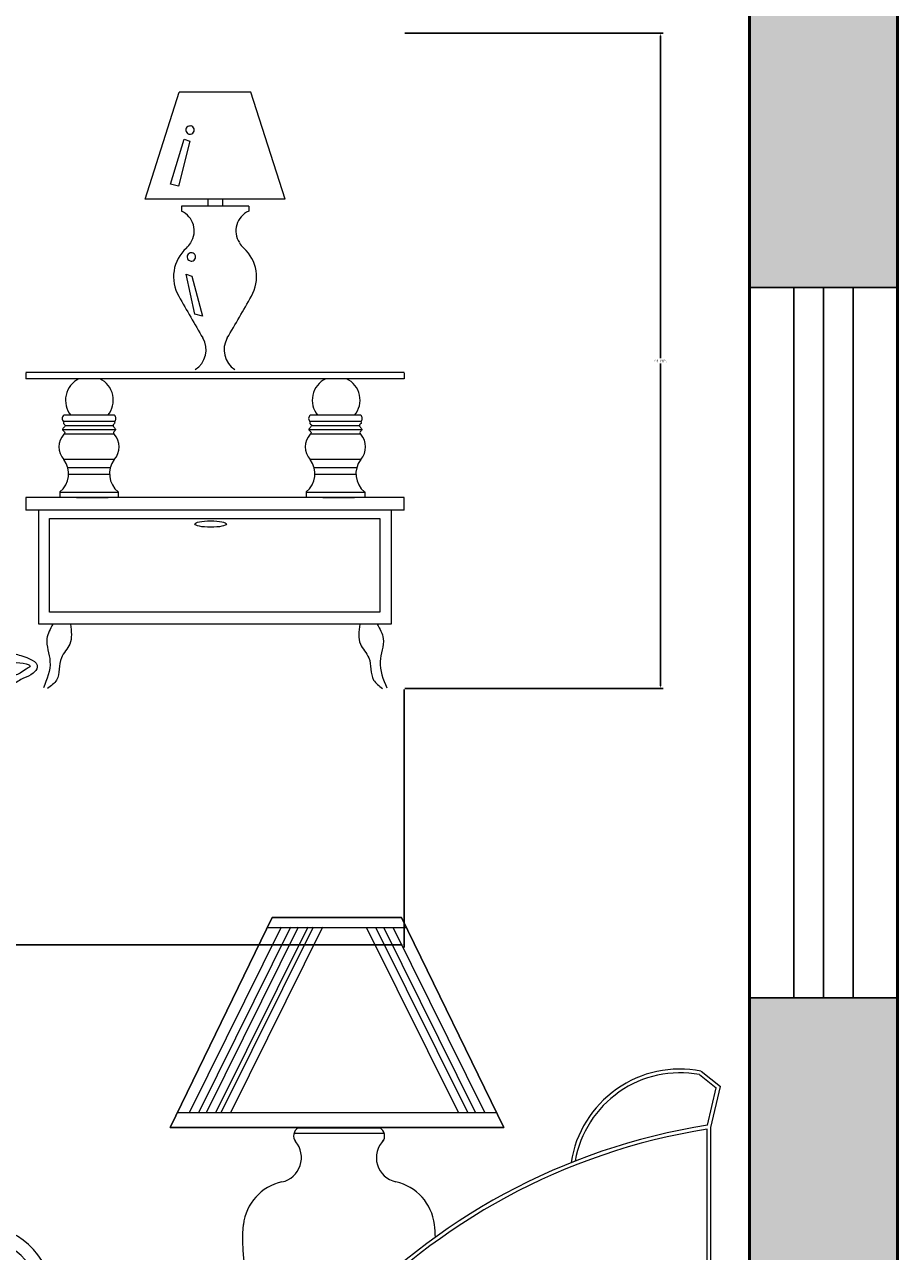
# Model space of a CAD drawing. Units: inches. Extents: x 1771 to 3025, y 319 to 889.
# Tile 23 of 35: x 2502 to 2561, y 703 to 786. Entities that reach past the tile are written whole.
import ezdxf

# ---------------------------------------------------------------- set-up
doc = ezdxf.new("R2010")
doc.units = ezdxf.units.IN
doc.header["$MEASUREMENT"] = 0
doc.set_wipeout_variables(frame=1)
for name, color, linetype, lineweight in [('A-ANNO-DIMS', 2, 'Continuous', 18), ('A-FURN', 8, 'Continuous', 18), ('A-GLAZ', 40, 'Continuous', 25), ('A-WALL', 7, 'Continuous', 50), ('A-WALL-PATT', 254, 'Continuous', 13)]:
    doc.layers.add(name, color=color, linetype=linetype, lineweight=lineweight)
doc.styles.get("Standard").update_dxf_attribs({"font": 'arial.ttf'})
doc.dimstyles.get("Standard").update_dxf_attribs({"dimtxt": 0.18, "dimasz": 0.18, "dimexe": 0.18, "dimexo": 0.0625, "dimgap": 0.09, "dimtad": 0, "dimtih": 1, "dimtoh": 1, "dimdec": 4, "dimzin": 0, "dimdsep": 46, "dimtxsty": 'Standard', "dimcen": 0.09, "dimadec": 0, "dimazin": 0, "dimtfac": 1, "dimtdec": 4, "dimtofl": 0, "dimtmove": 0, "dimatfit": 3, "dimfxl": 1, "dimtolj": 1, "dimtzin": 0, "dimarcsym": 0})

# ---------------------------------------------------------------- blocks, each defined once
blk = doc.blocks.new('A$C3F6F0378')
for p, q in [((2294.6, 774.2), (2348.7, 943.6)), ((2462.2, 943.6), (2348.7, 943.6)), ((2516.4, 774.2), (2462.2, 943.6)), ((2335.1, 797.8), (2356.3, 869.3)), ((2365.5, 866.2), (2347.3, 794.8)), ((2356.3, 869.3), (2365.5, 866.2)), ((2347.3, 794.8), (2335.1, 797.8)), ((2516.4, 774.2), (2294.6, 774.2)), ((2352.3, 763), (2352.3, 755.2)), ((2352.3, 763), (2352.3, 755.2)), ((2458.6, 763), (2352.3, 763)), ((2393.8, 774.2), (2393.8, 763)), ((2417.1, 763), (2393.8, 763)), ((2417.1, 774.2), (2417.1, 763)), ((2458.6, 763), (2458.6, 755.2)), ((2458.6, 763), (2458.6, 755.2)), ((2359.5, 655.6), (2368.6, 652.5)), ((2373.2, 592.3), (2359.5, 655.6)), ((2368.6, 652.5), (2385.4, 589.2)), ((2385.4, 589.2), (2373.2, 592.3)), ((2704.5, 500), (2106.1, 500)), ((2106.1, 499.7), (2106.1, 489.7)), ((2704.5, 490), (2106.1, 490)), ((2704.5, 499.7), (2704.5, 489.7)), ((2246.1, 432.2), (2166.1, 432.2)), ((2246.1, 432.2), (2166.1, 432.2)), ((2635.9, 432.2), (2555.9, 432.2)), ((2635.9, 432.2), (2555.9, 432.2)), ((2248, 409.3), (2164.1, 409.3)), ((2246.1, 422.2), (2166.1, 422.2)), ((2244.2, 415.4), (2167.9, 415.4)), ((2637.9, 409.3), (2554, 409.3)), ((2635.9, 422.2), (2555.9, 422.2)), ((2634.1, 415.4), (2557.7, 415.4)), ((2246.1, 402.2), (2166.1, 402.2)), ((2635.9, 402.2), (2555.9, 402.2)), ((2246.1, 362.2), (2166.1, 362.2)), ((2635.9, 362.2), (2555.9, 362.2)), ((2239.7, 349.2), (2172.4, 349.2)), ((2238.5, 338.7), (2173.6, 338.7)), ((2629.6, 349.2), (2562.2, 349.2)), ((2628.4, 338.7), (2563.5, 338.7)), ((2159.8, 311), (2159.8, 302.2)), ((2252.3, 311), (2252.3, 302.2)), ((2549.7, 311), (2549.7, 302.2)), ((2642.2, 311), (2642.2, 302.2)), ((2106.1, 302.2), (2106.1, 282.2)), ((2704.5, 302.2), (2106.1, 302.2)), ((2252.3, 310.3), (2159.8, 310.3)), ((2186.1, 302.2), (2226.1, 302.2)), ((2186.1, 302.2), (2236.1, 302.2)), ((2642.2, 310.3), (2549.7, 310.3)), ((2575.9, 302.2), (2615.9, 302.2)), ((2575.9, 302.2), (2625.9, 302.2)), ((2704.5, 282.2), (2704.5, 302.2)), ((2704.5, 282.2), (2106.1, 282.2)), ((2126.1, 282.2), (2126.1, 102.2)), ((2684.5, 102.2), (2684.5, 282.2)), ((2143.3, 268.9), (2666.3, 268.9)), ((2143.3, 120.8), (2143.3, 268.9)), ((2666.3, 268.9), (2666.3, 120.8)), ((2666.3, 120.8), (2143.3, 120.8)), ((2126.1, 102.2), (2684.5, 102.2))]:
    blk.add_line(p, q)
for centre, radius, start, end in [((2365.7, 883.6), 6.48, 168.6084, 233.2112), ((2365.7, 883.6), 6.49, 104.0344, 168.6084), ((2365.7, 883.5), 6.42, 233.2112, 255.9722), ((2366.1, 883.6), 6.51, 78.6968, 107.1924), ((2365.7, 883.8), 6.69, 255.9722, 278.2688), ((2365.7, 883.9), 6.81, 278.2688, 342.9026), ((2366.1, 883.7), 6.5, 50.1648, 78.6968), ((2366.2, 883.8), 6.35, 342.9026, 50.1648), ((2338.7, 724.1), 33.9, 326.6744, 66.3416), ((2472.2, 724.1), 33.9, 113.6584, 213.3256), ((2337, 722.3), 34.4, 312.0366, 330.6067), ((2473.8, 722.3), 34.4, 209.3933, 227.9634), ((2401.2, 651.2), 61.5, 132.0366, 209.8723), ((2367.7, 682.8), 6.48, 168.6084, 233.2112), ((2367.7, 682.8), 6.49, 104.0344, 168.6084), ((2368.1, 682.9), 6.51, 78.6968, 107.1924), ((2367.8, 683.1), 6.81, 278.2688, 342.9026), ((2368.1, 682.9), 6.5, 50.1648, 78.6968), ((2368.2, 683), 6.35, 342.9026, 50.1648), ((2409.6, 651.2), 61.5, 330.1277, 47.9634), ((2367.7, 682.8), 6.42, 233.2112, 255.9722), ((2367.8, 683), 6.69, 255.9722, 278.2688), ((11218.8, 5715.8), 10230.1, 209.87228, 210.29853), ((-6408, 5715.8), 10230.1, 329.70147, 330.12772), ((2353.9, 535.9), 37.3, 302.5427, 30.2985), ((2457, 535.9), 37.3, 149.7015, 237.4573), ((2206.6, 456.1), 37.8, 115.9414, 219.2084), ((2206.6, 456.1), 37.8, 320.7916, 64.0586), ((2597, 456.1), 37.8, 115.9414, 219.2084), ((2597, 456.1), 37.8, 320.7916, 64.0586), ((2169.8, 427.2), 6.24, 126.78, 233.22), ((2242.3, 427.2), 6.24, 306.78, 53.22), ((2559.7, 427.2), 6.24, 126.78, 233.22), ((2632.2, 427.2), 6.24, 306.78, 53.22), ((2188.1, 382.2), 29.7, 137.7452, 222.2548), ((2224, 382.2), 29.7, 317.7452, 42.2548), ((2577.9, 382.2), 29.7, 137.7452, 222.2548), ((2613.9, 382.2), 29.7, 317.7452, 42.2548), ((2136.7, 339.8), 37, 308.7547, 37.2668), ((2275.4, 339.8), 37, 142.7332, 231.2453), ((2526.5, 339.8), 37, 308.7547, 37.2668), ((2665.3, 339.8), 37, 142.7332, 231.2453)]:
    blk.add_arc(centre, radius, start, end)
blk.add_ellipse((2398.3, 260.1), major_axis=(25, 0), ratio=0.2)
for points, knots in [([(2166.1, 422.2), (2165.6, 421), (2164.6, 418.8), (2169.4, 417.1), (2166.2, 412.9), (2162.3, 408.7), (2169.1, 405.7), (2166.9, 403.1), (2166.1, 402.2)], [0, 0, 0, 0, 3.125, 6.207289, 10.622222, 14.901958, 20.470919, 23.596268, 23.596268, 23.596268, 23.596268]), ([(2246, 422.2), (2246.5, 421), (2247.5, 418.8), (2242.7, 417.1), (2245.9, 412.9), (2249.8, 408.7), (2243, 405.7), (2245.2, 403.1), (2246, 402.2)], [0, 0, 0, 0, 3.125, 6.207289, 10.622222, 14.901958, 20.470919, 23.596268, 23.596268, 23.596268, 23.596268]), ([(2555.9, 422.2), (2555.5, 421), (2554.5, 418.8), (2559.3, 417.1), (2556.1, 412.9), (2552.2, 408.7), (2559, 405.7), (2556.7, 403.1), (2555.9, 402.2)], [0, 0, 0, 0, 3.125, 6.207289, 10.622222, 14.901958, 20.470919, 23.596268, 23.596268, 23.596268, 23.596268]), ([(2635.9, 422.2), (2636.4, 421), (2637.3, 418.8), (2632.5, 417.1), (2635.8, 412.9), (2639.7, 408.7), (2632.8, 405.7), (2635.1, 403.1), (2635.9, 402.2)], [0, 0, 0, 0, 3.125, 6.207289, 10.622222, 14.901958, 20.470919, 23.596268, 23.596268, 23.596268, 23.596268]), ([(2148.9, 101.6), (2144.7, 94.2), (2134.2, 75.7), (2149.9, 40.1), (2139.4, 14.7), (2133.7, 0.9)], [0, 0, 0, 0, 24.696996, 61.099524, 104.177437, 104.177437, 104.177437, 104.177437]), ([(2176.5, 101.6), (2178, 90.6), (2180.7, 70.5), (2155.8, 47.4), (2161.8, 15.4), (2145.9, 4), (2140.4, 0)], [0, 0, 0, 0, 31.35672, 56.935761, 92.890491, 112.386558, 112.386558, 112.386558, 112.386558]), ([(2634.4, 101.6), (2632.9, 90.6), (2630.2, 70.5), (2655.1, 47.4), (2649.1, 15.4), (2665, 4), (2670.5, 0)], [0, 0, 0, 0, 31.35672, 56.935761, 92.890491, 112.386558, 112.386558, 112.386558, 112.386558]), ([(2662, 101.6), (2666.2, 94.2), (2676.7, 75.7), (2661, 40.1), (2671.5, 14.7), (2677.2, 0.9)], [0, 0, 0, 0, 24.696996, 61.099524, 104.177437, 104.177437, 104.177437, 104.177437])]:
    blk.add_open_spline(points, degree=3, knots=knots)
at = {"ltscale": 5}
for points, knots in [([(2084.9, 41.8), (2100.9, 40.1), (2120.5, 38.1), (2104.4, 29.7), (2095.5, 21.9), (2085.1, 19.8), (2078.6, 18.4)], [0, 0, 0, 0, 28.05485, 34.289435, 45.980108, 65.027556, 65.027556, 65.027556, 65.027556]), ([(2079, 57.4), (2084.9, 55.8), (2100.2, 51.8), (2131, 40.6), (2116.7, 21.1), (2101.3, 16.6), (2091, 9.7), (2085.5, 5.9)], [0, 0, 0, 0, 19.937155, 51.57724, 63.193909, 80.21631, 100.09061, 100.09061, 100.09061, 100.09061])]:
    blk.add_open_spline(points, degree=3, knots=knots, dxfattribs=at)
blk = doc.blocks.new('A$C425441F1')
for points in [[(1639.3, 0), (1667.3, 0), (1667.3, 55.3), (1748.6, 55.3), (1748.6, 807.4), (1761.1, 860.7), (1735.7, 880.7), (1703.4, 883.3), (1675.8, 879.6), (1656.2, 873.5), (1635.2, 863.3), (1619.6, 852.6), (1605.1, 839.5), (1596.7, 829.9), (1583.2, 810), (1573.2, 788.1), (1567.6, 767.7), (1566.5, 761.6), (1541.6, 750.9), (1510.7, 736.6), (1488.3, 725.3), (1464.5, 712.2), (1433.4, 693.6), (1409.1, 677.8), (1389.7, 664.2), (1388.2, 683.8), (1383.3, 700), (1376.2, 712), (1365.5, 723.2), (1352, 731.8), (1342.1, 735.4), (1331.7, 738.6), (1325, 742.7), (1317.7, 750.9), (1314.2, 758.8), (1312.9, 767.9), (1315.6, 780.8), (1321.1, 788.9), (1323.4, 793.7), (1323.6, 797.2), (1323.1, 800), (1320.5, 804.5), (1317.8, 806.7), (1317.8, 807.1), (1478.8, 807.1), (1345.8, 1080.7), (1177.3, 1080.7), (1044.3, 807.1), (1211.1, 807.1), (1211.1, 806.7), (1207.8, 803.9), (1205.8, 800.4), (1205.1, 796.3), (1207.6, 788.9), (1211.4, 783.4), (1213.5, 778.7), (1215.3, 769.8), (1215.1, 763.9), (1214.1, 759), (1208.8, 748.5), (1201.9, 741.7), (1195.3, 738), (1185.9, 735.4), (1176, 731.7), (1166.8, 726.4), (1159.9, 720.8), (1156.8, 717.7), (1149.3, 708.1), (1145.7, 701.6), (1143.6, 696.9), (1138.7, 669.7), (1138.7, 651.6), (1140.7, 631.8), (1142.6, 621.6), (1148.5, 600.5), (1162.8, 569), (1176.9, 547.8), (1188.6, 534.2), (1200, 523), (983, 523), (977.7, 522.3), (971.8, 519.6), (965.5, 512.8), (963.3, 506.8), (963, 503), (974.8, 503), (974.8, 3), (1013, 3), (1013, 103), (1053.6, 103), (1052.7, 96.1), (1051.6, 86.5), (1049.3, 63.6), (1048.6, 55.3), (1130.1, 55.3), (1130.1, 0), (1157.9, 0), (1174.1, 55.3), (1623.1, 55.6)], [(778.6, 0), (750.6, 0), (750.6, 50.4), (141.4, 50.4), (141.4, 0), (113.4, 0), (98.1, 50.4), (0, 50.4), (0, 590.4), (3.6, 609.1), (14.7, 633.7), (36.6, 658.7), (60.6, 673.3), (86.6, 680.5), (100.5, 681.5), (107.8, 698), (118.3, 717), (136.4, 751.3), (159.1, 779.5), (188.4, 803.6), (213.2, 817.4), (239.4, 827.1), (258.7, 831.4), (276, 833.4), (301.1, 842.1), (332.2, 850.9), (368.4, 858.6), (403.3, 863.5), (432.7, 865.8), (472.6, 866.2), (499.3, 864.8), (525, 862.1), (551.9, 857.9), (572.9, 853.6), (591.1, 849.1), (612.6, 842.8), (648, 830.4), (661.5, 823.7), (679.5, 815.2), (707.5, 798.2), (726.7, 783.3), (755.4, 754.4), (773.7, 729.8), (788.1, 704.9), (796.6, 686.1), (798.5, 681.2), (818, 677.9), (833.5, 672.3), (851.7, 661.6), (864.4, 650.3), (878.3, 632.1), (887.5, 611.7), (891.4, 595.2), (892, 590.4), (892, 50.4), (793.9, 50.4)]]:
    blk.add_wipeout(points)
for p, q in [((1044.3, 807.1), (1177.3, 1080.7)), ((1177.3, 1080.7), (1044.3, 807.1)), ((1177.3, 1080.7), (1345.8, 1080.7)), ((1345.8, 1080.7), (1177.3, 1080.7)), ((1345.8, 1080.7), (1478.8, 807.1)), ((1478.8, 807.1), (1345.8, 1080.7)), ((1188.8, 1068), (1069.3, 827.4)), ((1201.1, 1068), (1081.6, 827.4)), ((1211.2, 1068), (1091.7, 827.4)), ((1223.5, 1068), (1104, 827.4)), ((1230.5, 1068), (1110.9, 827.4)), ((1242.8, 1068), (1123.2, 827.4)), ((1171, 1067.8), (1351.9, 1067.8)), ((1299.6, 1068), (1419.2, 827.4)), ((1311.9, 1068), (1431.5, 827.4)), ((1322, 1068), (1441.5, 827.4)), ((1334.3, 1068), (1453.8, 827.4)), ((1735.7, 880.7), (1761.1, 860.7)), ((1733.6, 876.1), (1755.5, 858.7)), ((1744.1, 810.1), (1755.5, 858.7)), ((1748.6, 807.4), (1761.1, 860.7)), ((1053.8, 826.7), (1469.3, 826.7)), ((1478.8, 807.1), (1044.3, 807.1)), ((1044.3, 807.1), (1478.8, 807.1)), ((1205.6, 800), (1323.1, 800)), ((1211, 806.7), (1317.8, 806.7)), ((1743.6, 60.3), (1743.6, 805)), ((1748.6, 55.3), (1748.6, 807.4)), ((18.2, 603.6), (18.2, 536.8)), ((0, 590.4), (0, 50.4)), ((15, 591.1), (15, 521.6)), ((31, 569.9), (31, 588.4)), ((861, 569.9), (861, 588.4)), ((877, 591.1), (877, 521.6)), ((892, 590.4), (892, 50.4)), ((1238.2, 523), (983, 523)), ((1222, 503), (963, 503)), ((974.8, 3), (974.8, 503)), ((1206.8, 483), (974.8, 483)), ((1013, 3), (1013, 483)), ((10, 417.4), (32, 265.4)), ((882, 417.4), (860, 265.4)), ((1092.2, 423), (974.8, 423)), ((15, 385.1), (15, 50.4)), ((877, 385.1), (877, 50.4)), ((1055.6, 314.3), (1046.6, 240.3)), ((1060.1, 309.3), (1051.6, 239.7)), ((1111.1, 314.3), (1055.6, 314.3)), ((1109, 309.3), (1060.1, 309.3)), ((31, 50.4), (31, 272.3)), ((861, 50.4), (861, 272.3)), ((276.3, 240.8), (286.9, 216)), ((589.2, 240.9), (599.9, 216.1)), ((108.8, 209.4), (790.1, 209.4)), ((109.6, 209.4), (783, 209.4)), ((245.5, 223.1), (286.9, 216)), ((286.9, 216), (276.9, 175.2)), ((286.9, 216), (298.3, 173.5)), ((558.4, 223.2), (599.9, 216.1)), ((599.9, 216.1), (589.8, 175.3)), ((599.9, 216.1), (611.2, 173.6)), ((109.6, 199.4), (783, 199.4)), ((285.7, 179.9), (278.3, 201.7)), ((598.7, 180), (591.2, 201.8)), ((298.3, 173.5), (285.7, 179.9)), ((611.2, 173.6), (598.7, 180)), ((31.6, 128.4), (31.6, 131.4)), ((41.6, 128.4), (41.6, 131.4)), ((851, 131.4), (851, 128.4)), ((861, 131.4), (861, 128.4)), ((1056.5, 123), (1013, 123)), ((1053.6, 103), (1013, 103)), ((0, 50.4), (892, 50.4)), ((113.4, 0), (97.2, 53.4)), ((783, 60.4), (109.6, 60.4)), ((783, 50.4), (109.6, 50.4)), ((141.4, 50.4), (141.4, 0)), ((750.6, 50.4), (750.6, 0)), ((778.6, 0), (794.8, 53.4)), ((1048.6, 55.3), (1748.6, 55.3)), ((1054, 60.3), (1743.6, 60.3)), ((1129.9, 52.6), (1129.9, 0)), ((1157.9, 0), (1174.2, 55.6)), ((1639.3, 0), (1623.1, 55.6)), ((1667.3, 52.6), (1667.3, 0)), ((141.4, 0), (113.4, 0)), ((750.6, 0), (778.6, 0)), ((1129.9, 0), (1157.9, 0)), ((1667.3, 0), (1639.3, 0))]:
    blk.add_line(p, q)
for centre, radius, start, end in [((1708.4, 739.8), 143.6, 79.0486, 171.2543), ((458.1, 348.7), 517.8, 68.4843, 110.5916), ((1708.4, 739.8), 138.6, 79.5487, 170.0411), ((458.1, 348.7), 512.8, 68.4843, 110.5916), ((289.3, 651.4), 182.6, 93.9855, 176.965), ((289.3, 651.4), 177.6, 93.9855, 170.8791), ((563, 591.9), 246.9, 17.5917, 71.2419), ((563, 591.9), 251.9, 14.3659, 71.2419), ((1873.1, -6.5), 826.8, 98.9741, 175.711), ((1873.1, -6.5), 821.8, 99.0642, 175.3352), ((1217.2, 796.3), 12.1, 120.8914, 217.6223), ((1311.5, 796.3), 12.1, 322.3777, 59.1086), ((1183, 767.9), 32.3, 282.2329, 40.4775), ((1345.2, 767.9), 32.3, 135.1029, 257.7671), ((1203.5, 673.6), 64.2, 102.2329, 173.5671), ((1324.7, 673.6), 64.2, 6.4329, 77.7671), ((242.1, 635.9), 148, 144.2704, 189.5276), ((560.7, 643.7), 223.1, 296.1387, 23.9967), ((512.5, 645.7), 276.4, 357.4515, 12.4082), ((100.5, 580.5), 100.9, 89.5113, 174.4069), ((508.9, 316.7), 542.9, 139.0716, 146.5815), ((333.5, 586), 238.7, 156.9166, 219.7497), ((791.5, 580.5), 100.9, 5.5931, 89.1441), ((1322.1, 660.2), 183.7, 173.5671, 228.321), ((1206.1, 660.2), 183.7, 1.2452, 6.4329), ((104.5, 574.5), 91, 97.7735, 169.4907), ((316.8, 619.2), 213.4, 167.2983, 240.5749), ((331.3, 643.7), 223.1, 173.6107, 243.8613), ((383.1, 316.7), 542.9, 33.4185, 40.1113), ((787.5, 574.5), 91, 10.5093, 82.2265), ((104.5, 574.5), 74.8, 113.0142, 169.2704), ((787.5, 574.5), 74.8, 10.7296, 66.9858), ((579.4, 614.6), 207.2, 299.0365, 4.5654), ((578.1, 577), 217.9, 318.7723, 15.0106), ((301.8, 453.4), 294.8, 146.5815, 180), ((590.2, 453.4), 294.8, 0, 33.4185), ((983, 503), 20, 90, 180), ((56.7, 434.2), 49.4, 95.5103, 189.1585), ((48.3, 453.8), 40.5, 46.9039, 174.9451), ((49, 344.1), 139.3, 24.2628, 91.6479), ((843, 344.1), 139.3, 88.3521, 155.7372), ((843.7, 453.8), 40.5, 5.0549, 133.0961), ((835.3, 434.2), 49.4, 350.8415, 84.4897), ((1177.9, 391.7), 91.3, 73.3794, 227.0029), ((1177.9, 391.7), 86.3, 74.5383, 225.8439), ((301.8, 453.4), 294.8, 180, 193.379), ((468.1, -775.2), 1235.6, 77.9993, 104.2473), ((423.9, -775.2), 1235.6, 75.7527, 102.0007), ((590.2, 453.4), 294.8, 346.621, 0), ((52.4, 315.2), 153.2, 329.9033, 50.4478), ((839.6, 315.2), 153.2, 129.5522, 210.0967), ((92.5, 308.8), 126.8, 335.5815, 48.2351), ((799.5, 308.8), 126.8, 131.7649, 204.4185), ((114.7, 252.6), 85.8, 14.0074, 167.3648), ((135.5, 294.2), 81.5, 277.3995, 32.8179), ((756.5, 294.2), 81.5, 147.1821, 262.6005), ((777.3, 252.6), 85.8, 12.6352, 165.9926), ((106.2, 240.2), 87.4, 106.4444, 125.4727), ((114.5, 212.1), 116.8, 90, 106.4444), ((114.5, 212.1), 116.8, 73.5556, 90), ((122.8, 240.2), 87.4, 54.5273, 73.5556), ((769.2, 240.2), 87.4, 106.4444, 125.4727), ((777.5, 212.1), 116.8, 90, 106.4444), ((777.5, 212.1), 116.8, 73.5556, 90), ((785.8, 240.2), 87.4, 54.5273, 73.5556), ((93.5, 258.1), 65.5, 125.4727, 149.8309), ((135.5, 258.1), 65.5, 30.1691, 54.5273), ((756.5, 258.1), 65.5, 125.4727, 149.8309), ((798.5, 258.1), 65.5, 30.1691, 54.5273), ((74.1, 269.4), 43.1, 149.8309, 180), ((154.9, 269.4), 43.1, 0, 30.1691), ((737.1, 269.4), 43.1, 149.8309, 180), ((817.9, 269.4), 43.1, 0, 30.1691), ((74.1, 269.4), 43.1, 180, 210.1691), ((154.9, 269.4), 43.1, 329.8309, 0), ((737.1, 269.4), 43.1, 180, 210.1691), ((817.9, 269.4), 43.1, 329.8309, 0), ((93.5, 280.6), 65.5, 210.1691, 234.5273), ((135.5, 280.6), 65.5, 305.4727, 329.8309), ((756.5, 280.6), 65.5, 210.1691, 234.5273), ((798.5, 280.6), 65.5, 305.4727, 329.8309), ((1071.6, 237.3), 25.1, 173.0657, 279.7438), ((106.2, 298.5), 87.4, 234.5273, 253.5556), ((122.8, 298.5), 87.4, 286.4444, 305.4727), ((302.4, 220.7), 12.2, 53.3958, 216.551), ((615.4, 220.8), 12.2, 53.3958, 216.551), ((769.2, 298.5), 87.4, 234.5273, 253.5556), ((785.8, 298.5), 87.4, 286.4444, 305.4727), ((1071.6, 237.3), 20.1, 173.0657, 286.6808), ((109.6, 131.4), 78, 90, 180), ((114.5, 326.6), 116.8, 253.5556, 270), ((114.5, 326.6), 116.8, 270, 286.4444), ((294.4, 177.6), 35.9, 92.8846, 181.9), ((607.4, 177.7), 35.9, 92.8846, 181.9), ((777.5, 326.6), 116.8, 253.5556, 270), ((777.5, 326.6), 116.8, 270, 286.4444), ((783, 131.4), 78, 0, 90), ((109.6, 131.4), 68, 90, 180), ((783, 131.4), 68, 0, 90), ((271.5, 234.5), 59.6, 257.4358, 275.1883), ((584.4, 234.6), 59.6, 257.4358, 275.1883), ((109.6, 128.4), 78, 180, 270), ((109.6, 128.4), 68, 180, 270), ((783, 128.4), 68, 270, 0), ((783, 128.4), 78, 270, 0)]:
    blk.add_arc(centre, radius, start, end)
blk = doc.blocks.new('WIN-48')
for p, q in [((0, 0), (0, 10)), ((48, 0), (48, 10)), ((0, 7), (48, 7)), ((0, 5), (48, 5)), ((0, 3), (48, 3))]:
    blk.add_line(p, q)
blk = doc.blocks.new('*D36')
at = {"layer": 'A-ANNO-DIMS', "color": 0, "lineweight": -2, "transparency": 16777216}
for p, q in [((2412.284, 741.45), (2412.284, 724.003)), ((2527.809, 741.45), (2527.809, 724.003)), ((2412.464, 724.183), (2468.97, 724.183)), ((2527.629, 724.183), (2471.123, 724.183))]:
    blk.add_line(p, q, dxfattribs=at)
at = {"layer": 'A-ANNO-DIMS', "color": 0, "transparency": 16777216}
for points in [[(2412.464, 724.213), (2412.464, 724.153), (2412.284, 724.183)], [(2527.629, 724.213), (2527.629, 724.153), (2527.809, 724.183)]]:
    blk.add_solid(points, dxfattribs=at)
at = {"layer": 'Defpoints', "color": 0, "transparency": 16777216}
for p in [(2412.284, 741.512), (2527.809, 741.512), (2527.809, 724.183)]:
    blk.add_point(p, dxfattribs=at)
at = {"layer": 'A-ANNO-DIMS', "color": 0, "transparency": 16777216, "insert": (2470.046, 724.183), "char_height": 0.18, "attachment_point": 5}
blk.add_mtext('\\A1;BED B1 116 TYP.', dxfattribs=at)
blk = doc.blocks.new('*D37')
at = {"layer": 'A-ANNO-DIMS', "color": 0, "lineweight": -2, "transparency": 16777216}
for p, q in [((2527.871, 785.8), (2545.318, 785.8)), ((2545.138, 785.62), (2545.138, 763.836)), ((2545.138, 741.692), (2545.138, 763.476)), ((2527.871, 741.512), (2545.318, 741.512))]:
    blk.add_line(p, q, dxfattribs=at)
at = {"layer": 'A-ANNO-DIMS', "color": 0, "transparency": 16777216}
for points in [[(2545.108, 785.62), (2545.168, 785.62), (2545.138, 785.8)], [(2545.108, 741.692), (2545.168, 741.692), (2545.138, 741.512)]]:
    blk.add_solid(points, dxfattribs=at)
at = {"layer": 'Defpoints', "color": 0, "transparency": 16777216}
for p in [(2527.809, 785.8), (2545.138, 785.8), (2527.809, 741.512)]:
    blk.add_point(p, dxfattribs=at)
at = {"layer": 'A-ANNO-DIMS', "color": 0, "transparency": 16777216, "insert": (2545.138, 763.656), "char_height": 0.18, "attachment_point": 5}
blk.add_mtext('\\A1;44 TYP.', dxfattribs=at)

msp = doc.modelspace()

# ---------------------------------------------------------------- hatches: boundary and pattern name
at = {"layer": 'A-WALL-PATT'}
h = msp.add_hatch(color=256, dxfattribs=at)
h.dxf.hatch_style = 1
h.paths.add_polyline_path([(2407.162, 878.634), (2429.205, 878.634), (2429.205, 888.634), (2379.162, 888.634), (2379.162, 878.634), (2402.162, 878.634), (2402.162, 830.634), (2407.162, 830.634)])
h.paths.add_polyline_path([(2520.114, 888.634), (2477.205, 888.634), (2477.205, 878.634), (2498.162, 878.634), (2498.162, 794.634), (2402.162, 794.634), (2402.162, 758.634), (2402.162, 664.634), (2407.162, 664.634), (2407.162, 712), (2407.162, 789.634), (2515.162, 789.634), (2515.162, 794.634), (2503.162, 794.634), (2503.162, 878.634), (2520.114, 878.634)])
h.paths.add_polyline_path([(2561.162, 888.634), (2538.114, 888.634), (2538.114, 878.634), (2551.162, 878.634), (2551.162, 789.634), (2551.162, 768.608), (2561.162, 768.608)])
h.paths.add_polyline_path([(2561.162, 720.608), (2551.162, 720.608), (2551.162, 669.634), (2443.162, 669.634), (2443.162, 664.634), (2462.162, 664.634), (2462.162, 652.634), (2467.162, 652.634), (2467.162, 664.634), (2551.162, 664.634), (2551.162, 649.173), (2561.162, 649.173)])
h.paths.add_polyline_path([(2561.162, 631.173), (2551.162, 631.173), (2551.162, 616.634), (2462.162, 616.634), (2443.162, 616.634), (2443.162, 611.634), (2551.162, 611.634), (2551.162, 581.106), (2561.162, 581.106)])
h.paths.add_polyline_path([(2561.162, 533.106), (2551.162, 533.106), (2551.162, 479.634), (2407.162, 479.634), (2407.162, 616.634), (2397.162, 616.634), (2397.162, 543.634), (2306.162, 543.634), (2306.162, 533.634), (2397.162, 533.634), (2397.162, 469.634), (2551.162, 469.634), (2551.162, 452.762), (2561.162, 452.762)])
h.paths.add_polyline_path([(2561.162, 404.762), (2551.162, 404.762), (2551.162, 393.634), (2397.162, 393.634), (2397.162, 383.634), (2561.162, 383.634)])
h.paths.add_polyline_path([(2270.162, 642.584), (2260.162, 642.584), (2260.162, 533.634), (2270.162, 533.634)])
h.paths.add_polyline_path([(2270.162, 753.634), (2366.162, 753.634), (2366.162, 758.634), (2270.162, 758.634), (2270.162, 842.589, -0.008336), (2268.859, 842.634), (2260.162, 842.634), (2260.162, 690.584), (2270.162, 690.584)])
h.paths.add_polyline_path([(2331.162, 888.634), (2260.162, 888.634), (2260.162, 878.634), (2331.162, 878.634)])

# ---------------------------------------------------------------- linework, layer by layer
at = {"layer": 'A-WALL'}
for p, q in [((2561.162, 383.634), (2561.162, 888.432)), ((2551.162, 669.634), (2551.162, 789.634))]:
    msp.add_line(p, q, dxfattribs=at)

# ---------------------------------------------------------------- block references
at = {"layer": 'A-FURN', "xscale": 0.0427162254345911, "yscale": 0.0427162254345911, "zscale": 0.0427162254345911}
msp.add_blockref('A$C3F6F0378', (2412.284, 741.512), dxfattribs=at)
at = {"layer": 'A-GLAZ', "rotation": 270.0000000000007}
msp.add_blockref('WIN-48', (2551.162, 768.608), dxfattribs=at)

# ---------------------------------------------------------------- dimensions: what is measured, and where the dimension line sits
at = {"layer": 'A-ANNO-DIMS'}
dim = msp.add_linear_dim(base=(2545.138, 785.8), p1=(2527.809, 741.512), p2=(2527.809, 785.8), angle=90, text='<> TYP.', dimstyle='Standard', override={"dimdec": 0, "dimrnd": 0, "dimzin": 0, "dimlunit": 2}, dxfattribs=at)
dim.commit()
dim.dimension.update_dxf_attribs({"geometry": '*D37', "text_midpoint": (2545.138, 763.656)})

# ---------------------------------------------------------------- next in the draw order: block references
at = {"layer": 'A-FURN', "xscale": 0.0519011286993662, "yscale": 0.0519011286993662, "zscale": 0.0519011286993662}
msp.add_blockref('A$C425441F1', (2457.798, 669.938), dxfattribs=at)

# ---------------------------------------------------------------- next in the draw order: dimensions: what is measured, and where the dimension line sits
at = {"layer": 'A-ANNO-DIMS'}
dim = msp.add_linear_dim(base=(2527.809, 724.183), p1=(2412.284, 741.512), p2=(2527.809, 741.512), text='BED B1 <> TYP.', dimstyle='Standard', override={"dimdec": 0, "dimrnd": 0, "dimzin": 0, "dimlunit": 2}, dxfattribs=at)
dim.commit()
dim.dimension.update_dxf_attribs({"geometry": '*D36', "text_midpoint": (2470.046, 724.183)})

doc.saveas('drawing.dxf')
